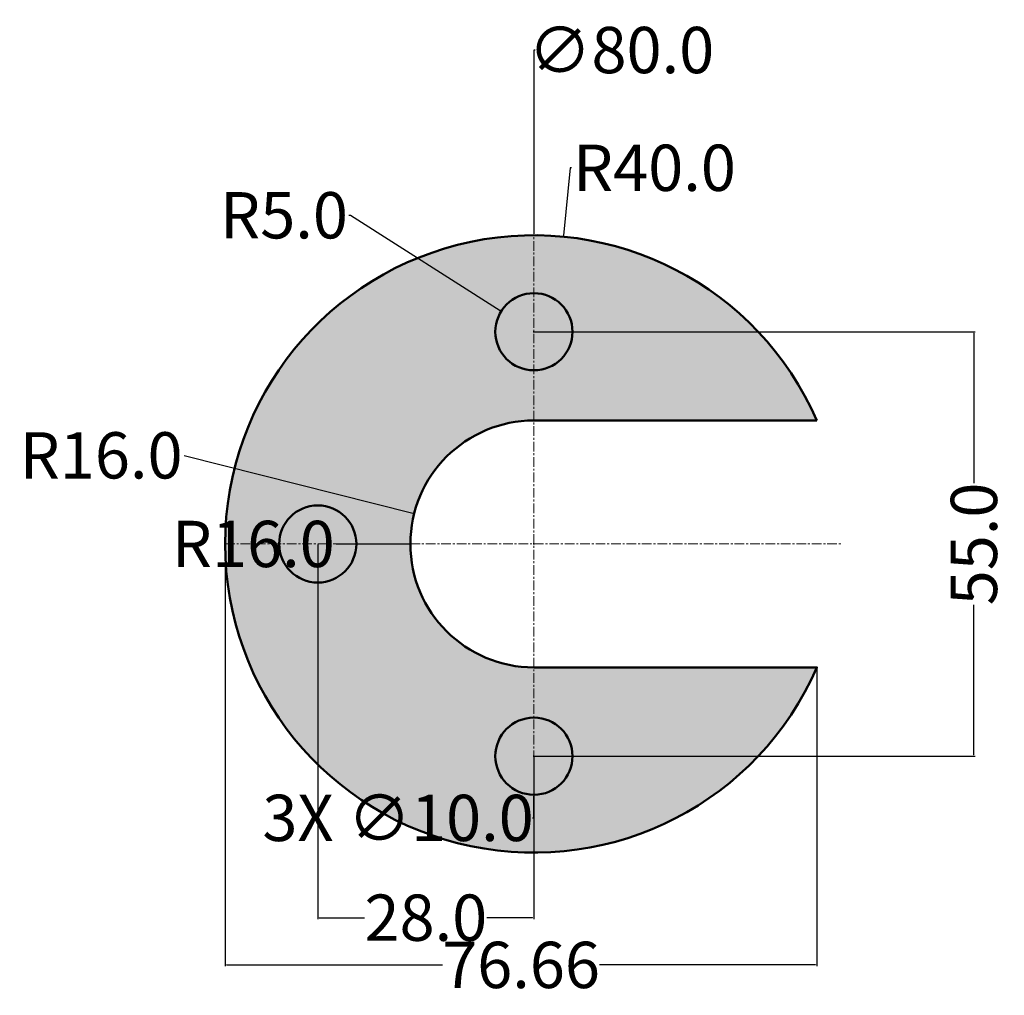
# Model space of a CAD drawing. Units: millimetres. Extents: x 0 to 127, y 10 to 137.
import ezdxf

# ---------------------------------------------------------------- set-up
doc = ezdxf.new("R2010")
doc.units = ezdxf.units.MM
doc.header["$MEASUREMENT"] = 0
doc.linetypes.add('CENTER', pattern=[2, 1.25, -0.25, 0.25, -0.25])
for name, color, linetype, lineweight in [('M-CNTR', 4, 'CENTER', 18), ('M-DIMS', 2, 'Continuous', 25), ('M-HATC', 8, 'Continuous', 18), ('M-OUTL', 7, 'Continuous', 50)]:
    doc.layers.add(name, color=color, linetype=linetype, lineweight=lineweight)
doc.styles.get("Standard").update_dxf_attribs({"font": 'arial.ttf'})
doc.dimstyles.get("Standard").update_dxf_attribs({"dimtxt": 6, "dimasz": 0.18, "dimexe": 0.18, "dimexo": 0.0625, "dimgap": 0.09, "dimtad": 0, "dimtoh": 1, "dimdec": 1, "dimzin": 0, "dimdsep": 46, "dimtxsty": 'Standard', "dimcen": 0.09, "dimadec": 0, "dimazin": 0, "dimtfac": 1, "dimtdec": 1, "dimtofl": 0, "dimtmove": 0, "dimatfit": 3, "dimfxl": 1, "dimtolj": 1, "dimtzin": 0, "dimarcsym": 0})

# ---------------------------------------------------------------- blocks, each defined once
blk = doc.blocks.new('*D1')
at = {"layer": 'Defpoints', "color": 0, "transparency": 16777216}
for p in [(66.37, 96.41), (66.37, 41.41), (123.36, 41.41)]:
    blk.add_point(p, dxfattribs=at)
at = {"layer": 'M-DIMS', "color": 0, "lineweight": -2, "transparency": 16777216}
for p, q in [((66.43, 96.41), (123.54, 96.41)), ((123.36, 96.23), (123.36, 76.78)), ((123.36, 41.59), (123.36, 61.03)), ((66.43, 41.41), (123.54, 41.41))]:
    blk.add_line(p, q, dxfattribs=at)
at = {"layer": 'M-DIMS', "color": 0, "transparency": 16777216}
for points in [[(123.33, 96.23), (123.39, 96.23), (123.36, 96.41)], [(123.33, 41.59), (123.39, 41.59), (123.36, 41.41)]]:
    blk.add_solid(points, dxfattribs=at)
at = {"layer": 'M-DIMS', "color": 0, "transparency": 16777216, "insert": (123.36, 68.91), "char_height": 6, "attachment_point": 5, "rotation": 90}
blk.add_mtext('\\A1;55.0', dxfattribs=at)
blk = doc.blocks.new('*D2')
at = {"layer": 'Defpoints', "color": 0, "transparency": 16777216}
for p in [(38.37, 68.91), (66.37, 41.41), (38.37, 20.48)]:
    blk.add_point(p, dxfattribs=at)
at = {"layer": 'M-DIMS', "color": 0, "lineweight": -2, "transparency": 16777216}
for p, q in [((38.37, 68.84), (38.37, 20.3)), ((66.37, 41.34), (66.37, 20.3)), ((38.55, 20.48), (44.44, 20.48)), ((66.19, 20.48), (60.29, 20.48))]:
    blk.add_line(p, q, dxfattribs=at)
at = {"layer": 'M-DIMS', "color": 0, "transparency": 16777216}
for points in [[(38.55, 20.51), (38.55, 20.45), (38.37, 20.48)], [(66.19, 20.51), (66.19, 20.45), (66.37, 20.48)]]:
    blk.add_solid(points, dxfattribs=at)
at = {"layer": 'M-DIMS', "color": 0, "transparency": 16777216, "insert": (52.37, 20.48), "char_height": 6, "attachment_point": 5}
blk.add_mtext('\\A1;28.0', dxfattribs=at)
blk = doc.blocks.new('*D3')
at = {"layer": 'Defpoints', "color": 0, "transparency": 16777216}
for p in [(50.86, 72.84), (66.37, 68.91)]:
    blk.add_point(p, dxfattribs=at)
at = {"layer": 'M-DIMS', "color": 0, "lineweight": -2, "transparency": 16777216}
for p, q in [((21.05, 80.39), (50.68, 72.88)), ((66.28, 68.91), (66.46, 68.91)), ((66.37, 68.82), (66.37, 69))]:
    blk.add_line(p, q, dxfattribs=at)
at = {"layer": 'M-DIMS', "color": 0, "transparency": 16777216}
blk.add_solid([(50.69, 72.91), (50.67, 72.85), (50.86, 72.84)], dxfattribs=at)
at = {"layer": 'M-DIMS', "color": 0, "transparency": 16777216, "insert": (10.31, 80.39), "char_height": 6, "attachment_point": 5}
blk.add_mtext('\\A1;R16.0', dxfattribs=at)
blk = doc.blocks.new('*D4')
at = {"layer": 'Defpoints', "color": 0, "transparency": 16777216}
for p in [(70.2, 108.72), (66.37, 68.91)]:
    blk.add_point(p, dxfattribs=at)
at = {"layer": 'M-DIMS', "color": 0, "lineweight": -2, "transparency": 16777216}
for p, q in [((71.05, 117.65), (70.21, 108.9)), ((71.23, 117.65), (71.05, 117.65)), ((66.28, 68.91), (66.46, 68.91)), ((66.37, 68.82), (66.37, 69))]:
    blk.add_line(p, q, dxfattribs=at)
at = {"layer": 'M-DIMS', "color": 0, "transparency": 16777216}
blk.add_solid([(70.18, 108.91), (70.24, 108.9), (70.2, 108.72)], dxfattribs=at)
at = {"layer": 'M-DIMS', "color": 0, "transparency": 16777216, "insert": (81.98, 117.65), "char_height": 6, "attachment_point": 5}
blk.add_mtext('\\A1;R40.0', dxfattribs=at)
blk = doc.blocks.new('*D5')
at = {"layer": 'Defpoints', "color": 0, "transparency": 16777216}
for p in [(62.15, 99.09), (66.37, 96.41)]:
    blk.add_point(p, dxfattribs=at)
at = {"layer": 'M-DIMS', "color": 0, "lineweight": -2, "transparency": 16777216}
for p, q in [((42.41, 111.5), (42.59, 111.5)), ((42.59, 111.5), (61.99, 99.18)), ((66.28, 96.41), (66.46, 96.41)), ((66.37, 96.32), (66.37, 96.5))]:
    blk.add_line(p, q, dxfattribs=at)
at = {"layer": 'M-DIMS', "color": 0, "transparency": 16777216}
blk.add_solid([(62.01, 99.21), (61.98, 99.16), (62.15, 99.09)], dxfattribs=at)
at = {"layer": 'M-DIMS', "color": 0, "transparency": 16777216, "insert": (34, 111.5), "char_height": 6, "attachment_point": 5}
blk.add_mtext('\\A1;R5.0', dxfattribs=at)
blk = doc.blocks.new('HOLE-D10')
blk.add_circle((5, 5), 5)
blk = doc.blocks.new('*D7')
at = {"layer": 'Defpoints', "color": 0, "transparency": 16777216}
for p in [(26.37, 68.91), (103.03, 52.91), (103.03, 14.36)]:
    blk.add_point(p, dxfattribs=at)
at = {"layer": 'M-DIMS', "color": 0, "lineweight": -2, "transparency": 16777216}
for p, q in [((26.37, 68.84), (26.37, 14.18)), ((103.03, 52.84), (103.03, 14.18)), ((26.55, 14.36), (54.51, 14.36)), ((102.85, 14.36), (74.88, 14.36))]:
    blk.add_line(p, q, dxfattribs=at)
at = {"layer": 'M-DIMS', "color": 0, "transparency": 16777216}
for points in [[(26.55, 14.39), (26.55, 14.33), (26.37, 14.36)], [(102.85, 14.39), (102.85, 14.33), (103.03, 14.36)]]:
    blk.add_solid(points, dxfattribs=at)
at = {"layer": 'M-DIMS', "color": 0, "transparency": 16777216, "insert": (64.7, 14.36), "char_height": 6, "attachment_point": 5}
blk.add_mtext('\\A1;76.66', dxfattribs=at)
blk = doc.blocks.new('*D8')
at = {"layer": 'Defpoints', "color": 0, "transparency": 16777216}
for p in [(66.37, 108.91), (66.37, 28.91)]:
    blk.add_point(p, dxfattribs=at)
at = {"layer": 'M-DIMS', "color": 0, "lineweight": -2, "transparency": 16777216}
for p, q in [((66.55, 132.91), (66.37, 132.91)), ((66.37, 132.91), (66.37, 109.09)), ((66.28, 68.91), (66.46, 68.91)), ((66.37, 68.82), (66.37, 69))]:
    blk.add_line(p, q, dxfattribs=at)
at = {"layer": 'M-DIMS', "color": 0, "transparency": 16777216}
blk.add_solid([(66.34, 109.09), (66.4, 109.09), (66.37, 108.91)], dxfattribs=at)
at = {"layer": 'M-DIMS', "color": 0, "transparency": 16777216, "insert": (77.68, 132.91), "char_height": 6, "attachment_point": 5}
blk.add_mtext('\\A1;∅80.0', dxfattribs=at)
blk = doc.blocks.new('*D9')
at = {"layer": 'Defpoints', "color": 0, "transparency": 16777216}
for p in [(50.37, 68.91), (66.37, 68.91)]:
    blk.add_point(p, dxfattribs=at)
at = {"layer": 'M-DIMS', "color": 0, "lineweight": -2, "transparency": 16777216}
for p, q in [((40.77, 68.91), (50.19, 68.91)), ((66.28, 68.91), (66.46, 68.91)), ((66.37, 68.82), (66.37, 69))]:
    blk.add_line(p, q, dxfattribs=at)
at = {"layer": 'M-DIMS', "color": 0, "transparency": 16777216}
blk.add_solid([(50.19, 68.94), (50.19, 68.88), (50.37, 68.91)], dxfattribs=at)
at = {"layer": 'M-DIMS', "color": 0, "transparency": 16777216, "insert": (30.02, 68.91), "char_height": 6, "attachment_point": 5}
blk.add_mtext('\\A1;R16.0', dxfattribs=at)
blk = doc.blocks.new('*D10')
at = {"layer": 'Defpoints', "color": 0, "transparency": 16777216}
for p in [(66.37, 46.41), (66.37, 36.41)]:
    blk.add_point(p, dxfattribs=at)
at = {"layer": 'M-DIMS', "color": 0, "lineweight": -2, "transparency": 16777216}
for p, q in [((66.28, 41.41), (66.46, 41.41)), ((66.37, 41.32), (66.37, 41.5)), ((66.37, 33.41), (66.37, 36.23)), ((66.19, 33.41), (66.37, 33.41))]:
    blk.add_line(p, q, dxfattribs=at)
at = {"layer": 'M-DIMS', "color": 0, "transparency": 16777216}
blk.add_solid([(66.34, 36.23), (66.4, 36.23), (66.37, 36.41)], dxfattribs=at)
at = {"layer": 'M-DIMS', "color": 0, "transparency": 16777216, "insert": (48.77, 33.41), "char_height": 6, "attachment_point": 5}
blk.add_mtext('\\A1;3X ∅10.0', dxfattribs=at)

msp = doc.modelspace()

# ---------------------------------------------------------------- hatches: boundary and pattern name
at = {"layer": 'M-HATC'}
h = msp.add_hatch(color=256, dxfattribs=at)
h.set_gradient(color1=(242, 103, 34), color2=(255, 255, 0), tint=1, name='CYLINDER')
h.paths.add_polyline_path([(66.366, 91.407, -0.4142136), (61.366, 96.407, -0.4142136), (66.366, 101.407), (66.366, 108.907, 0.4142136), (26.366, 68.907), (33.366, 68.907, -1), (43.366, 68.907), (50.366, 68.907, -0.4142136), (66.366, 84.907)])
h.paths.add_polyline_path([(66.366, 108.907), (66.366, 101.407, -0.4142136), (71.366, 96.407, -0.4142136), (66.366, 91.407), (66.366, 84.907), (103.027, 84.907, 0.2982166)])
h.paths.add_polyline_path([(50.366, 68.907), (43.366, 68.907, -1), (33.366, 68.907), (26.366, 68.907, 0.4142136), (66.366, 28.907), (66.366, 36.407, -0.4142136), (61.366, 41.407, -0.4142136), (66.366, 46.407), (66.366, 52.907, -0.4142136)])
h.paths.add_polyline_path([(103.027, 52.907), (66.366, 52.907), (66.366, 46.407, -0.4142136), (71.366, 41.407, -0.4142136), (66.366, 36.407), (66.366, 28.907, 0.2982166)])
h = msp.add_hatch(color=256, dxfattribs=at)
h.set_gradient(color1=(0, 255, 255), color2=(0, 255, 255), tint=1, name='CYLINDER')
h.paths.add_polyline_path([(66.366, 101.407, 0.4142136), (61.366, 96.407, 0.4142136), (66.366, 91.407)])
h.paths.add_polyline_path([(66.366, 101.407), (66.366, 91.407, 0.4142136), (71.366, 96.407, 0.4142136)])
h.paths.add_polyline_path([(33.366, 68.907), (43.366, 68.907, 1)])
h.paths.add_polyline_path([(43.366, 68.907), (33.366, 68.907, 1)])
h.paths.add_polyline_path([(66.366, 46.407, 0.4142136), (61.366, 41.407, 0.4142136), (66.366, 36.407)])
h.paths.add_polyline_path([(66.366, 46.407), (66.366, 36.407, 0.4142136), (71.366, 41.407, 0.4142136)])

# ---------------------------------------------------------------- linework, layer by layer
at = {"layer": 'M-CNTR'}
for p, q in [((66.366, 28.907), (66.366, 108.907)), ((26.366, 68.907), (106.366, 68.907))]:
    msp.add_line(p, q, dxfattribs=at)
at = {"layer": 'M-OUTL'}
msp.add_lwpolyline([(103.027, 84.907), (66.366, 84.907, 1), (66.366, 52.907), (103.027, 52.907, -4.7912878)], format="xyb", close=True, dxfattribs=at)

# ---------------------------------------------------------------- block references
for p in [(61.366, 91.407), (33.366, 63.907), (61.366, 36.407)]:
    msp.add_blockref('HOLE-D10', p, dxfattribs=at)

# ---------------------------------------------------------------- dimensions: what is measured, and where the dimension line sits
at = {"layer": 'M-DIMS'}
dim = msp.add_diameter_dim_2p(p1=(66.366, 28.907), p2=(66.366, 108.907), dimstyle='Standard', override={"dimdec": 1, "dimlfac": 1, "dimrnd": 0, "dimzin": 0, "dimdsep": 46, "dimlunit": 2}, dxfattribs=at)
dim.commit()
dim.dimension.update_dxf_attribs({"geometry": '*D8', "text_midpoint": (77.682, 132.907), "dimtype": 163})
for center, mpoint, override, picture, middle in [((66.366, 68.907), (70.195, 108.724), {"dimclrd": 0, "dimclre": 0, "dimclrt": 0}, '*D4', (81.977, 117.649)), ((66.366, 96.407), (62.145, 99.088), {"dimclrd": 0, "dimclre": 0, "dimclrt": 0}, '*D5', (34, 111.504)), ((66.366, 68.907), (50.857, 72.839), {"dimclrd": 0, "dimclre": 0, "dimclrt": 0}, '*D3', (21.054, 80.393)), ((66.366, 68.907), (50.366, 68.907), {"dimdec": 1, "dimlfac": 1, "dimrnd": 0, "dimzin": 0, "dimdsep": 46, "dimlunit": 2}, '*D9', (40.766, 68.907))]:
    dim = msp.add_radius_dim(center=center, mpoint=mpoint, dimstyle='Standard', override=override, dxfattribs=at)
    dim.commit()
    dim.dimension.update_dxf_attribs({"geometry": picture, "text_midpoint": middle, "dimtype": 164})
dim = msp.add_linear_dim(base=(123.36, 41.407), p1=(66.366, 96.407), p2=(66.366, 41.407), angle=90, dimstyle='Standard', override={"dimclrd": 0, "dimclre": 0, "dimclrt": 0}, dxfattribs=at)
dim.commit()
dim.dimension.update_dxf_attribs({"geometry": '*D1', "text_midpoint": (123.36, 68.907)})
for base, p1, p2, override, picture, middle in [((103.027, 14.357), (26.366, 68.907), (103.027, 52.907), {"dimdec": 2, "dimlfac": 1, "dimrnd": 0, "dimzin": 0, "dimdsep": 46, "dimlunit": 2}, '*D7', (64.696, 14.357)), ((38.366, 20.477), (66.366, 41.407), (38.366, 68.907), {"dimclrd": 0, "dimclre": 0, "dimclrt": 0}, '*D2', (52.366, 20.477))]:
    dim = msp.add_linear_dim(base=base, p1=p1, p2=p2, dimstyle='Standard', override=override, dxfattribs=at)
    dim.commit()
    dim.dimension.update_dxf_attribs({"geometry": picture, "text_midpoint": middle})
dim = msp.add_diameter_dim_2p(p1=(66.366, 46.407), p2=(66.366, 36.407), text='3X <>', dimstyle='Standard', override={"dimdec": 1, "dimlfac": 1, "dimrnd": 0, "dimzin": 0, "dimdsep": 46, "dimlunit": 2}, dxfattribs=at)
dim.commit()
dim.dimension.update_dxf_attribs({"geometry": '*D10', "text_midpoint": (48.765, 33.407), "dimtype": 163})

doc.saveas('drawing.dxf')
